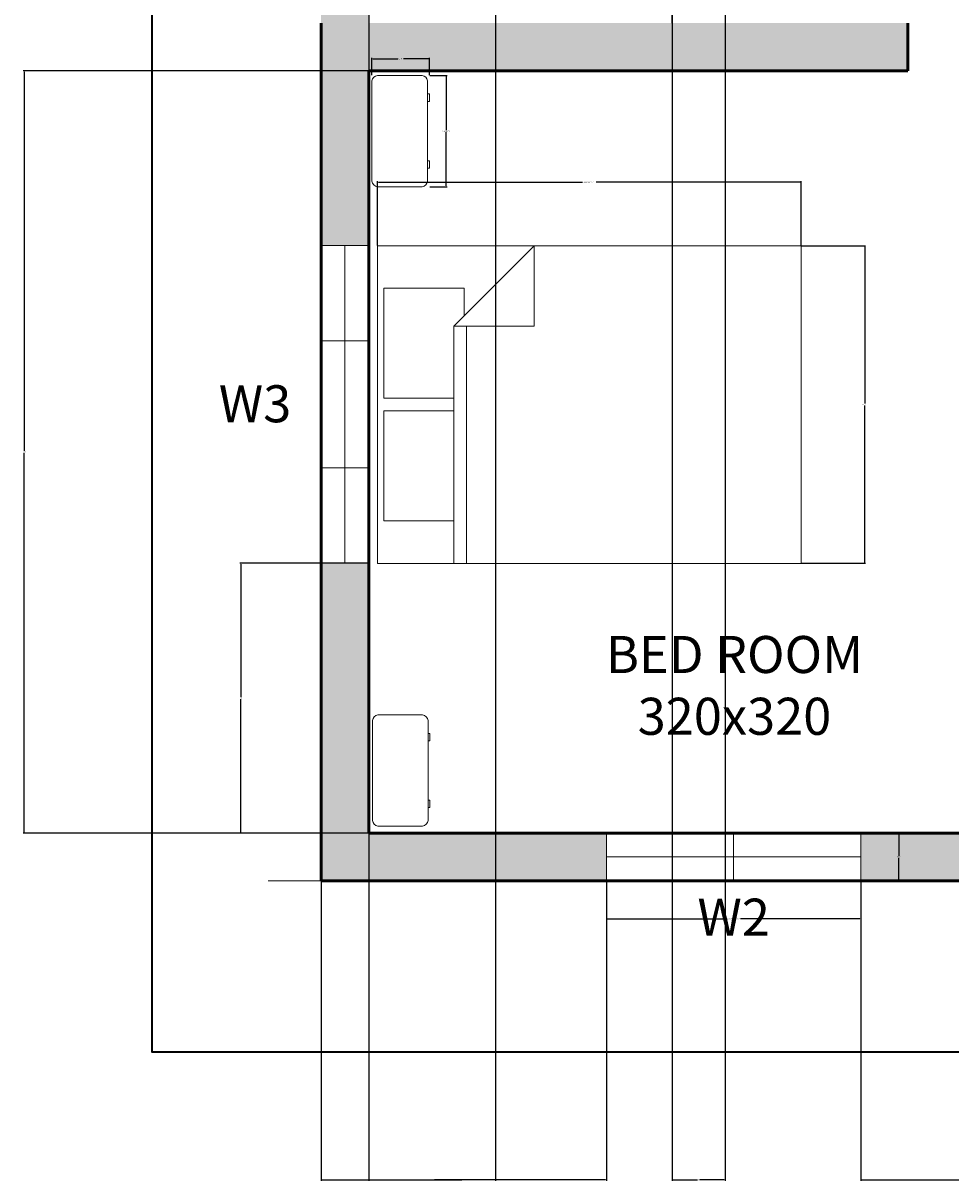
# Model space of a CAD drawing. Units: inches. Extents: x 5191 to 5616, y 7031 to 7539.
# Tile 1 of 4: x 5191 to 5367, y 7031 to 7250. Entities that reach past the tile are written whole.
import ezdxf

# ---------------------------------------------------------------- set-up
doc = ezdxf.new("R2010")
doc.units = ezdxf.units.IN
for name, color, linetype, lineweight in [('A-ANNO-DIMS', 2, 'Continuous', 13), ('A-ANNO-TEXT', 7, 'Continuous', 18), ('A-ANNO-TTLB', 7, 'Continuous', 35), ('A-AREA-IDEN', 7, 'Continuous', 25), ('A-FLOR-STRS', 7, 'Continuous', 25), ('A-FURN', 8, 'Continuous', 18), ('A-GLAZ', 4, 'Continuous', 18), ('A-WALL', 7, 'Continuous', 50)]:
    doc.layers.add(name, color=color, linetype=linetype, lineweight=lineweight)
doc.layers.add('A-WALL-PATT', color=177, linetype='Continuous', lineweight=13, true_color=0x293189)
doc.styles.get("Standard").update_dxf_attribs({"font": 'arial.ttf'})
doc.dimstyles.get("Standard").update_dxf_attribs({"dimtxt": 0.18, "dimasz": 0.18, "dimexe": 0.18, "dimexo": 0.0625, "dimgap": 0.09, "dimtad": 0, "dimtih": 1, "dimtoh": 1, "dimdec": 4, "dimzin": 0, "dimdsep": 46, "dimtxsty": 'Standard', "dimcen": 0.09, "dimadec": 0, "dimazin": 0, "dimtfac": 1, "dimtdec": 4, "dimtofl": 0, "dimtmove": 0, "dimatfit": 3, "dimfxl": 1, "dimtolj": 1, "dimtzin": 0, "dimarcsym": 0})

# ---------------------------------------------------------------- blocks, each defined once
blk = doc.blocks.new('Bed - Queen')
for p, q in [((0, -80.00003), (0, 0)), ((0, 0), (59.99999, 0)), ((59.99999, 0), (59.99999, -80.00003)), ((7.99999, -1.2), (28.79998, -1.2)), ((7.99999, -14.4), (7.99999, -1.2)), ((28.79998, -1.2), (28.79998, -14.4)), ((31.19999, -1.2), (51.99999, -1.2)), ((31.19999, -14.4), (31.19999, -1.2)), ((51.99999, -1.2), (51.99999, -16.4)), ((0, -14.4), (44.8, -14.4)), ((59.99999, -29.6), (44.8, -14.4)), ((44.8, -14.4), (44.8, -29.6)), ((44.8, -16.8), (0, -16.8)), ((51.99999, -16.4), (46.79936, -16.4)), ((44.8, -29.6), (59.99999, -29.6)), ((59.99999, -80.00003), (0, -80.00003))]:
    blk.add_line(p, q)
blk = doc.blocks.new('Desk - 30 x 60 in.')
for p, q in [((-26.999995, 0), (26.999995, 0)), ((-29.999995, -27), (-29.999995, -3)), ((29.999995, -3), (29.999995, -27)), ((26.999995, -30), (-26.999995, -30)), ((-20.000005, -30), (-20.000005, -31)), ((-20.000005, -31), (-16.000005, -31)), ((-16.000005, -31), (-16.000005, -30)), ((15.999995, -31), (15.999995, -30)), ((19.999995, -31), (15.999995, -31)), ((19.999995, -30), (19.999995, -31))]:
    blk.add_line(p, q)
for centre, start, end in [((-26.499995, -3.5), 98.1301, 171.8699), ((26.499995, -3.5), 8.130102, 81.8699), ((-26.499995, -26.5), 188.1301, 261.8699), ((26.499995, -26.5), 278.1301, 351.8699)]:
    blk.add_arc(centre, 3.535534, start, end)
blk = doc.blocks.new('WIN-W2-48IN')
for p, q in [((0, 0), (0, 9)), ((24, 0), (24, 9)), ((48, 0), (48, 9)), ((0, 4.5), (48, 4.5))]:
    blk.add_line(p, q)
blk = doc.blocks.new('WIN-W3-60IN')
for p, q in [((9, 60), (0, 60)), ((4.5, 60), (4.5, 0)), ((9, 42), (0, 42)), ((9, 18), (0, 18)), ((9, 0), (0, 0))]:
    blk.add_line(p, q)
blk = doc.blocks.new('*D13')
at = {"layer": 'A-ANNO-DIMS', "color": 0, "lineweight": -2, "transparency": 16777216}
for p, q in [((5268.16, 7239.74), (5271.43, 7239.74)), ((5271.25, 7239.56), (5271.25, 7229.41)), ((5271.25, 7218.9), (5271.25, 7229.05)), ((5268.16, 7218.72), (5271.43, 7218.72))]:
    blk.add_line(p, q, dxfattribs=at)
at = {"layer": 'A-ANNO-DIMS', "color": 0, "transparency": 16777216}
for points in [[(5271.22, 7239.56), (5271.28, 7239.56), (5271.25, 7239.74)], [(5271.22, 7218.9), (5271.28, 7218.9), (5271.25, 7218.72)]]:
    blk.add_solid(points, dxfattribs=at)
at = {"layer": 'Defpoints', "color": 0, "transparency": 16777216}
for p in [(5268.09, 7239.74), (5271.25, 7239.74), (5268.09, 7218.72)]:
    blk.add_point(p, dxfattribs=at)
at = {"layer": 'A-ANNO-DIMS', "color": 0, "transparency": 16777216, "insert": (5271.25, 7229.23), "char_height": 0.18, "attachment_point": 5}
blk.add_mtext('\\A1;DESK 21 TYP.', dxfattribs=at)
blk = doc.blocks.new('*D14')
at = {"layer": 'A-ANNO-DIMS', "color": 0, "lineweight": -2, "transparency": 16777216}
for p, q in [((5257.23, 7239.8), (5257.23, 7243.07)), ((5257.41, 7242.89), (5262.14, 7242.89)), ((5267.91, 7242.89), (5263.18, 7242.89)), ((5268.09, 7239.8), (5268.09, 7243.07))]:
    blk.add_line(p, q, dxfattribs=at)
at = {"layer": 'A-ANNO-DIMS', "color": 0, "transparency": 16777216}
for points in [[(5257.41, 7242.92), (5257.41, 7242.86), (5257.23, 7242.89)], [(5267.91, 7242.92), (5267.91, 7242.86), (5268.09, 7242.89)]]:
    blk.add_solid(points, dxfattribs=at)
at = {"layer": 'Defpoints', "color": 0, "transparency": 16777216}
for p in [(5257.23, 7242.89), (5257.23, 7239.74), (5268.09, 7239.74)]:
    blk.add_point(p, dxfattribs=at)
at = {"layer": 'A-ANNO-DIMS', "color": 0, "transparency": 16777216, "insert": (5262.66, 7242.89), "char_height": 0.18, "attachment_point": 5}
blk.add_mtext('\\A1;11 TYP.', dxfattribs=at)
blk = doc.blocks.new('*D15')
at = {"layer": 'A-ANNO-DIMS', "color": 0, "lineweight": -2, "transparency": 16777216}
for p, q in [((5301.51, 7087.55), (5301.51, 7080.23)), ((5349.51, 7087.55), (5349.51, 7080.23)), ((5301.69, 7080.41), (5324.17, 7080.41)), ((5349.33, 7080.41), (5326.85, 7080.41))]:
    blk.add_line(p, q, dxfattribs=at)
at = {"layer": 'A-ANNO-DIMS', "color": 0, "transparency": 16777216}
for points in [[(5301.69, 7080.44), (5301.69, 7080.38), (5301.51, 7080.41)], [(5349.33, 7080.44), (5349.33, 7080.38), (5349.51, 7080.41)]]:
    blk.add_solid(points, dxfattribs=at)
at = {"layer": 'Defpoints', "color": 0, "transparency": 16777216}
for p in [(5301.51, 7087.61), (5349.51, 7087.61), (5349.51, 7080.41)]:
    blk.add_point(p, dxfattribs=at)
at = {"layer": 'A-ANNO-DIMS', "color": 0, "transparency": 16777216, "insert": (5325.51, 7080.41), "char_height": 0.18, "attachment_point": 5}
blk.add_mtext('\\A1;WINDOW W2 48 TYP.', dxfattribs=at)
blk = doc.blocks.new('*D16')
at = {"layer": 'A-ANNO-DIMS', "color": 0, "lineweight": -2, "transparency": 16777216}
for p, q in [((5349.57, 7096.61), (5356.89, 7096.61)), ((5356.71, 7096.43), (5356.71, 7092.3)), ((5356.71, 7087.79), (5356.71, 7091.93)), ((5349.57, 7087.61), (5356.89, 7087.61))]:
    blk.add_line(p, q, dxfattribs=at)
at = {"layer": 'A-ANNO-DIMS', "color": 0, "transparency": 16777216}
for points in [[(5356.68, 7096.43), (5356.74, 7096.43), (5356.71, 7096.61)], [(5356.68, 7087.79), (5356.74, 7087.79), (5356.71, 7087.61)]]:
    blk.add_solid(points, dxfattribs=at)
at = {"layer": 'Defpoints', "color": 0, "transparency": 16777216}
for p in [(5349.51, 7096.61), (5356.71, 7096.61), (5349.51, 7087.61)]:
    blk.add_point(p, dxfattribs=at)
at = {"layer": 'A-ANNO-DIMS', "color": 0, "transparency": 16777216, "insert": (5356.71, 7092.11), "char_height": 0.18, "attachment_point": 5}
blk.add_mtext('\\A1;9 TYP.', dxfattribs=at)
blk = doc.blocks.new('*D19')
at = {"layer": 'A-ANNO-DIMS', "color": 0, "lineweight": -2, "transparency": 16777216}
for p, q in [((5258.27, 7207.63), (5258.27, 7219.75)), ((5258.45, 7219.57), (5296.97, 7219.57)), ((5338.09, 7219.57), (5299.57, 7219.57)), ((5338.27, 7207.63), (5338.27, 7219.75))]:
    blk.add_line(p, q, dxfattribs=at)
at = {"layer": 'A-ANNO-DIMS', "color": 0, "transparency": 16777216}
for points in [[(5258.45, 7219.6), (5258.45, 7219.54), (5258.27, 7219.57)], [(5338.09, 7219.6), (5338.09, 7219.54), (5338.27, 7219.57)]]:
    blk.add_solid(points, dxfattribs=at)
at = {"layer": 'Defpoints', "color": 0, "transparency": 16777216}
for p in [(5258.27, 7219.57), (5258.27, 7207.57), (5338.27, 7207.57)]:
    blk.add_point(p, dxfattribs=at)
at = {"layer": 'A-ANNO-DIMS', "color": 0, "transparency": 16777216, "insert": (5298.27, 7219.57), "char_height": 0.18, "attachment_point": 5}
blk.add_mtext('\\A1;QUEEN BED 80 TYP.', dxfattribs=at)
blk = doc.blocks.new('*D20')
at = {"layer": 'A-ANNO-DIMS', "color": 0, "lineweight": -2, "transparency": 16777216}
for p, q in [((5338.33, 7207.57), (5350.45, 7207.57)), ((5350.27, 7207.39), (5350.27, 7177.75)), ((5350.27, 7147.75), (5350.27, 7177.39)), ((5338.33, 7147.57), (5350.45, 7147.57))]:
    blk.add_line(p, q, dxfattribs=at)
at = {"layer": 'A-ANNO-DIMS', "color": 0, "transparency": 16777216}
for points in [[(5350.24, 7207.39), (5350.3, 7207.39), (5350.27, 7207.57)], [(5350.24, 7147.75), (5350.3, 7147.75), (5350.27, 7147.57)]]:
    blk.add_solid(points, dxfattribs=at)
at = {"layer": 'Defpoints', "color": 0, "transparency": 16777216}
for p in [(5338.27, 7207.57), (5350.27, 7207.57), (5338.27, 7147.57)]:
    blk.add_point(p, dxfattribs=at)
at = {"layer": 'A-ANNO-DIMS', "color": 0, "transparency": 16777216, "insert": (5350.27, 7177.57), "char_height": 0.18, "attachment_point": 5}
blk.add_mtext('\\A1;60 TYP.', dxfattribs=at)
blk = doc.blocks.new('*D33')
at = {"layer": 'A-ANNO-DIMS', "color": 0, "lineweight": -2, "transparency": 16777216}
for p, q in [((5247.63, 7087.55), (5247.63, 7030.92)), ((5301.51, 7087.55), (5301.51, 7030.92)), ((5247.81, 7031.1), (5274.18, 7031.1)), ((5301.33, 7031.1), (5274.96, 7031.1))]:
    blk.add_line(p, q, dxfattribs=at)
at = {"layer": 'A-ANNO-DIMS', "color": 0, "transparency": 16777216}
for points in [[(5247.81, 7031.13), (5247.81, 7031.07), (5247.63, 7031.1)], [(5301.33, 7031.13), (5301.33, 7031.07), (5301.51, 7031.1)]]:
    blk.add_solid(points, dxfattribs=at)
at = {"layer": 'Defpoints', "color": 0, "transparency": 16777216}
for p in [(5247.63, 7087.61), (5301.51, 7087.61), (5301.51, 7031.1)]:
    blk.add_point(p, dxfattribs=at)
at = {"layer": 'A-ANNO-DIMS', "color": 0, "transparency": 16777216, "insert": (5274.57, 7031.1), "char_height": 0.18, "attachment_point": 5}
blk.add_mtext('\\A1;53.88', dxfattribs=at)
blk = doc.blocks.new('*D34')
at = {"layer": 'A-ANNO-DIMS', "color": 0, "lineweight": -2, "transparency": 16777216}
for p, q in [((5349.51, 7087.55), (5349.51, 7030.92)), ((5403.39, 7087.55), (5403.39, 7030.92)), ((5349.69, 7031.1), (5376.06, 7031.1)), ((5403.21, 7031.1), (5376.84, 7031.1))]:
    blk.add_line(p, q, dxfattribs=at)
at = {"layer": 'A-ANNO-DIMS', "color": 0, "transparency": 16777216}
for points in [[(5349.69, 7031.13), (5349.69, 7031.07), (5349.51, 7031.1)], [(5403.21, 7031.13), (5403.21, 7031.07), (5403.39, 7031.1)]]:
    blk.add_solid(points, dxfattribs=at)
at = {"layer": 'Defpoints', "color": 0, "transparency": 16777216}
for p in [(5349.51, 7087.61), (5403.39, 7087.61), (5403.39, 7031.1)]:
    blk.add_point(p, dxfattribs=at)
at = {"layer": 'A-ANNO-DIMS', "color": 0, "transparency": 16777216, "insert": (5376.45, 7031.1), "char_height": 0.18, "attachment_point": 5}
blk.add_mtext('\\A1;53.88', dxfattribs=at)
blk = doc.blocks.new('*D39')
at = {"layer": 'A-ANNO-DIMS', "color": 0, "lineweight": -2, "transparency": 16777216}
for p, q in [((5256.57, 7240.61), (5191.41, 7240.61)), ((5191.59, 7240.43), (5191.59, 7168.79)), ((5191.59, 7096.79), (5191.59, 7168.43)), ((5256.57, 7096.61), (5191.41, 7096.61))]:
    blk.add_line(p, q, dxfattribs=at)
at = {"layer": 'A-ANNO-DIMS', "color": 0, "transparency": 16777216}
for points in [[(5191.56, 7240.43), (5191.62, 7240.43), (5191.59, 7240.61)], [(5191.56, 7096.79), (5191.62, 7096.79), (5191.59, 7096.61)]]:
    blk.add_solid(points, dxfattribs=at)
at = {"layer": 'Defpoints', "color": 0, "transparency": 16777216}
for p in [(5191.59, 7240.61), (5256.63, 7240.61), (5256.63, 7096.61)]:
    blk.add_point(p, dxfattribs=at)
at = {"layer": 'A-ANNO-DIMS', "color": 0, "transparency": 16777216, "insert": (5191.59, 7168.61), "char_height": 0.18, "attachment_point": 5}
blk.add_mtext('\\A1;144', dxfattribs=at)
blk = doc.blocks.new('*D58')
at = {"layer": 'A-ANNO-DIMS', "color": 0, "lineweight": -2, "transparency": 16777216}
for p, q in [((5256.57, 7147.61), (5232.3, 7147.61)), ((5232.48, 7147.43), (5232.48, 7122.3)), ((5232.48, 7096.79), (5232.48, 7121.93)), ((5256.57, 7096.61), (5232.3, 7096.61))]:
    blk.add_line(p, q, dxfattribs=at)
at = {"layer": 'A-ANNO-DIMS', "color": 0, "transparency": 16777216}
for points in [[(5232.45, 7147.43), (5232.51, 7147.43), (5232.48, 7147.61)], [(5232.45, 7096.79), (5232.51, 7096.79), (5232.48, 7096.61)]]:
    blk.add_solid(points, dxfattribs=at)
at = {"layer": 'Defpoints', "color": 0, "transparency": 16777216}
for p in [(5232.48, 7147.61), (5256.63, 7147.61), (5256.63, 7096.61)]:
    blk.add_point(p, dxfattribs=at)
at = {"layer": 'A-ANNO-DIMS', "color": 0, "transparency": 16777216, "insert": (5232.48, 7122.11), "char_height": 0.18, "attachment_point": 5}
blk.add_mtext('\\A1;51', dxfattribs=at)
blk = doc.blocks.new('*D59')
at = {"layer": 'A-ANNO-DIMS', "color": 0, "lineweight": -2, "transparency": 16777216}
for p, q in [((5313.91, 7328.27), (5313.91, 7030.92)), ((5323.91, 7328.27), (5323.91, 7030.92)), ((5314.09, 7031.1), (5318.7, 7031.1)), ((5323.73, 7031.1), (5319.12, 7031.1))]:
    blk.add_line(p, q, dxfattribs=at)
at = {"layer": 'A-ANNO-DIMS', "color": 0, "transparency": 16777216}
for points in [[(5314.09, 7031.13), (5314.09, 7031.07), (5313.91, 7031.1)], [(5323.73, 7031.13), (5323.73, 7031.07), (5323.91, 7031.1)]]:
    blk.add_solid(points, dxfattribs=at)
at = {"layer": 'Defpoints', "color": 0, "transparency": 16777216}
for p in [(5313.91, 7328.33), (5323.91, 7328.33), (5323.91, 7031.1)]:
    blk.add_point(p, dxfattribs=at)
at = {"layer": 'A-ANNO-DIMS', "color": 0, "transparency": 16777216, "insert": (5318.91, 7031.1), "char_height": 0.18, "attachment_point": 5}
blk.add_mtext('\\A1;10', dxfattribs=at)
blk = doc.blocks.new('*D64')
at = {"layer": 'A-ANNO-DIMS', "color": 0, "lineweight": -2, "transparency": 16777216}
for p, q in [((5256.63, 7485.71), (5256.63, 7030.92)), ((5280.54, 7452.44), (5280.54, 7030.92)), ((5256.81, 7031.1), (5268.12, 7031.1)), ((5280.36, 7031.1), (5269.05, 7031.1))]:
    blk.add_line(p, q, dxfattribs=at)
at = {"layer": 'A-ANNO-DIMS', "color": 0, "transparency": 16777216}
for points in [[(5256.81, 7031.13), (5256.81, 7031.07), (5256.63, 7031.1)], [(5280.36, 7031.13), (5280.36, 7031.07), (5280.54, 7031.1)]]:
    blk.add_solid(points, dxfattribs=at)
at = {"layer": 'Defpoints', "color": 0, "transparency": 16777216}
for p in [(5256.63, 7485.77), (5280.54, 7452.51), (5280.54, 7031.1)]:
    blk.add_point(p, dxfattribs=at)
at = {"layer": 'A-ANNO-DIMS', "color": 0, "transparency": 16777216, "insert": (5268.59, 7031.1), "char_height": 0.18, "attachment_point": 5}
blk.add_mtext('\\A1;23.913', dxfattribs=at)

msp = doc.modelspace()

# ---------------------------------------------------------------- hatches: boundary and pattern name
at = {"layer": 'A-WALL-PATT'}
h = msp.add_hatch(color=256, dxfattribs=at)
h.dxf.hatch_style = 1
h.paths.add_polyline_path([(5297.311, 7494.7733), (5247.631, 7494.7733), (5247.631, 7441.5533), (5256.631, 7441.5533), (5256.631, 7485.7733), (5297.311, 7485.7733)])
h.paths.add_polyline_path([(5503.471, 7430.6933), (5503.471, 7461.7733), (5494.471, 7461.7733), (5494.471, 7430.6933), (5430.991, 7430.6933), (5430.991, 7485.7733), (5450.731, 7485.7733), (5450.731, 7494.7733), (5421.991, 7494.7733), (5421.991, 7485.7733), (5421.991, 7337.3333), (5421.991, 7328.3333), (5430.991, 7328.3333), (5430.991, 7337.3333), (5430.991, 7421.6933), (5503.471, 7421.6933)])
h.paths.add_polyline_path([(5385.991, 7494.7733), (5345.311, 7494.7733), (5345.311, 7485.7733), (5385.991, 7485.7733)])
h.paths.add_polyline_path([(5558.071, 7494.7733), (5474.731, 7494.7733), (5474.731, 7485.7733), (5494.471, 7485.7733), (5503.471, 7485.7733), (5549.071, 7485.7733), (5549.071, 7397.3333), (5558.071, 7397.3333)])
h.paths.add_polyline_path([(5385.991, 7337.3333), (5256.631, 7337.3333), (5256.631, 7381.5533), (5247.631, 7381.5533), (5247.631, 7337.3333), (5247.631, 7328.3333), (5247.631, 7300.9733), (5256.631, 7300.9733), (5256.631, 7328.3333), (5385.991, 7328.3333)])
h.paths.add_polyline_path([(5358.391, 7249.6133), (5303.911, 7249.6133), (5256.631, 7249.6133), (5256.631, 7276.9733), (5247.631, 7276.9733), (5247.631, 7249.6133), (5247.631, 7240.6133), (5247.631, 7207.6133), (5256.631, 7207.6133), (5256.631, 7240.6133), (5303.911, 7240.6133), (5358.391, 7240.6133)])
h.paths.add_polyline_path([(5256.631, 7114.6133), (5256.631, 7147.6133), (5247.631, 7147.6133), (5247.631, 7114.6133), (5247.631, 7105.6133), (5247.631, 7087.6133), (5301.511, 7087.6133), (5301.511, 7096.6133), (5256.631, 7096.6133)])
h.paths.add_polyline_path([(5403.391, 7105.6133), (5403.391, 7114.6133), (5403.391, 7134.8933), (5412.4598, 7134.8933), (5412.4598, 7143.8933), (5403.391, 7143.8933), (5403.391, 7249.6133), (5394.391, 7249.6133), (5394.391, 7143.8933), (5394.391, 7134.8933), (5394.391, 7114.6133), (5394.391, 7096.6133), (5349.511, 7096.6133), (5349.511, 7087.6133), (5403.391, 7087.6133)])
h.paths.add_polyline_path([(5558.071, 7143.8933), (5558.071, 7186.7933), (5549.071, 7186.7933), (5549.071, 7143.8933), (5527.2654, 7143.8933), (5527.2654, 7134.8933), (5558.071, 7134.8933)])
h.paths.add_polyline_path([(5479.2654, 7143.8933), (5448.4598, 7143.8933), (5448.4598, 7134.8933), (5479.2654, 7134.8933)])
h.paths.add_polyline_path([(5558.071, 7337.3333), (5549.071, 7337.3333), (5549.071, 7286.6933), (5421.991, 7286.6933), (5421.991, 7277.6933), (5430.991, 7277.6933), (5549.071, 7277.6933), (5549.071, 7234.7933), (5558.071, 7234.7933), (5558.071, 7277.6933)])

# ---------------------------------------------------------------- linework, layer by layer
at = {"layer": 'A-ANNO-DIMS'}
for q in [(5237.631, 7087.6133), (5247.631, 7077.6133)]:
    msp.add_line((5247.631, 7087.6133), q, dxfattribs=at)
at = {"layer": 'A-ANNO-TTLB'}
msp.add_lwpolyline([(5215.7388, 7536.9841), (5591.3795, 7536.9841), (5591.3795, 7055.2452), (5215.7388, 7055.2452)], close=True, dxfattribs=at)
at = {"layer": 'A-FLOR-STRS'}
msp.add_line((5313.911, 7249.6133), (5313.911, 7328.3333), dxfattribs=at)
at = {"layer": 'A-WALL'}
for p, q in [((5247.631, 7249.6133), (5247.631, 7240.6133)), ((5358.391, 7249.6133), (5358.391, 7240.6133)), ((5247.631, 7240.6133), (5247.631, 7114.6133)), ((5256.631, 7240.6133), (5303.911, 7240.6133)), ((5256.631, 7240.6133), (5256.631, 7114.6133)), ((5303.911, 7240.6133), (5358.391, 7240.6133)), ((5247.631, 7114.6133), (5247.631, 7105.6133)), ((5256.631, 7114.6133), (5256.631, 7096.6133)), ((5247.631, 7105.6133), (5247.631, 7087.6133)), ((5394.391, 7096.6133), (5256.631, 7096.6133)), ((5403.391, 7087.6133), (5247.631, 7087.6133))]:
    msp.add_line(p, q, dxfattribs=at)

# ---------------------------------------------------------------- block references
at = {"layer": 'A-FURN', "xscale": 0.350301795417789, "yscale": 0.350301795417789, "zscale": 0.350301795417789, "rotation": 89.99999999999999}
for p in [(5257.2336, 7229.2318), (5257.3174, 7108.4226)]:
    msp.add_blockref('Desk - 30 x 60 in.', p, dxfattribs=at)
at = {"layer": 'A-FURN', "rotation": 89.99999999999999}
msp.add_blockref('Bed - Queen', (5258.2698, 7147.5671), dxfattribs=at)
at = {"layer": 'A-GLAZ', "rotation": 180}
msp.add_blockref('WIN-W3-60IN', (5256.631, 7207.6136), dxfattribs=at)
at = {"layer": 'A-GLAZ'}
msp.add_blockref('WIN-W2-48IN', (5301.511, 7087.613), dxfattribs=at)

# ---------------------------------------------------------------- texts
at = {"layer": 'A-ANNO-TEXT', "char_height": 7, "attachment_point": 1}
for s, insert in [('\\pxqc;W3', (5220.3074, 7181.2161)), ('\\pxqc;W2', (5310.6824, 7084.2287))]:
    msp.add_mtext_dynamic_manual_height_columns(s, width=29.703042, gutter_width=12.5, heights=[0], dxfattribs=dict(at, insert=insert))
at = {"layer": 'A-AREA-IDEN', "insert": (5279.3872, 7133.8436), "char_height": 7, "attachment_point": 1}
msp.add_mtext_dynamic_manual_height_columns('\\pxqc;{\\fArial|b1|i0|c0|p34;BED ROOM\\P320x320}', width=92.590487, gutter_width=12.5, heights=[0], dxfattribs=at)

# ---------------------------------------------------------------- dimensions: what is measured, and where the dimension line sits
at = {"layer": 'A-ANNO-DIMS'}
for base, p1, p2, override, picture, middle in [((5280.5439, 7031.0952), (5256.631, 7485.7733), (5280.5439, 7452.5072), {"dimdec": 3, "dimlfac": 1, "dimrnd": 0, "dimzin": 0, "dimdsep": 46, "dimlunit": 2}, '*D64', (5268.5874, 7031.0952)), ((5323.911, 7031.0952), (5313.911, 7328.3333), (5323.911, 7328.3333), {"dimdec": 0, "dimlfac": 1, "dimrnd": 0, "dimzin": 0, "dimdsep": 46, "dimlunit": 2}, '*D59', (5318.911, 7031.0952)), ((5301.511, 7031.0952), (5247.631, 7087.6133), (5301.511, 7087.6133), {"dimdec": 2, "dimlfac": 1, "dimrnd": 0, "dimzin": 0, "dimdsep": 46, "dimlunit": 2}, '*D33', (5274.571, 7031.0952)), ((5403.391, 7031.0952), (5349.511, 7087.6133), (5403.391, 7087.6133), {"dimdec": 2, "dimlfac": 1, "dimrnd": 0, "dimzin": 0, "dimdsep": 46, "dimlunit": 2}, '*D34', (5376.451, 7031.0952))]:
    dim = msp.add_linear_dim(base=base, p1=p1, p2=p2, dimstyle='Standard', override=override, dxfattribs=at)
    dim.commit()
    dim.dimension.update_dxf_attribs({"geometry": picture, "text_midpoint": middle})
for base, p1, p2, angle, text, picture, middle in [((5257.2336, 7242.8936), (5268.0929, 7239.7409), (5257.2336, 7239.7409), 180, '<> TYP.', '*D14', (5262.6632, 7242.8936)), ((5271.2456, 7239.7409), (5268.0929, 7218.7228), (5268.0929, 7239.7409), 90, 'DESK <> TYP.', '*D13', (5271.2456, 7229.2318)), ((5258.2698, 7219.5671), (5338.2698, 7207.5671), (5258.2698, 7207.5671), 180, 'QUEEN BED <> TYP.', '*D19', (5298.2698, 7219.5671)), ((5350.2698, 7207.5671), (5338.2698, 7147.5671), (5338.2698, 7207.5671), 90, '<> TYP.', '*D20', (5350.2698, 7177.5671)), ((5356.711, 7096.6133), (5349.511, 7087.6133), (5349.511, 7096.6133), 90, '<> TYP.', '*D16', (5356.711, 7092.1133))]:
    dim = msp.add_linear_dim(base=base, p1=p1, p2=p2, angle=angle, text=text, dimstyle='Standard', override={"dimdec": 0, "dimlfac": 1, "dimrnd": 0, "dimzin": 0, "dimdsep": 46, "dimlunit": 2}, dxfattribs=at)
    dim.commit()
    dim.dimension.update_dxf_attribs({"geometry": picture, "text_midpoint": middle})
for base, p2, picture, middle in [((5191.5888, 7240.6133), (5256.631, 7240.6133), '*D39', (5191.5888, 7168.6133)), ((5232.481, 7147.6133), (5256.631, 7147.6133), '*D58', (5232.481, 7122.1133))]:
    dim = msp.add_linear_dim(base=base, p1=(5256.631, 7096.6133), p2=p2, angle=90, dimstyle='Standard', override={"dimdec": 0, "dimlfac": 1, "dimrnd": 0, "dimzin": 0, "dimdsep": 46, "dimlunit": 2}, dxfattribs=at)
    dim.commit()
    dim.dimension.update_dxf_attribs({"geometry": picture, "text_midpoint": middle})
dim = msp.add_linear_dim(base=(5349.511, 7080.4133), p1=(5301.511, 7087.6133), p2=(5349.511, 7087.6133), text='WINDOW W2 <> TYP.', dimstyle='Standard', override={"dimdec": 0, "dimlfac": 1, "dimrnd": 0, "dimzin": 0, "dimdsep": 46, "dimlunit": 2}, dxfattribs=at)
dim.commit()
dim.dimension.update_dxf_attribs({"geometry": '*D15', "text_midpoint": (5325.511, 7080.4133)})

doc.saveas('drawing.dxf')
